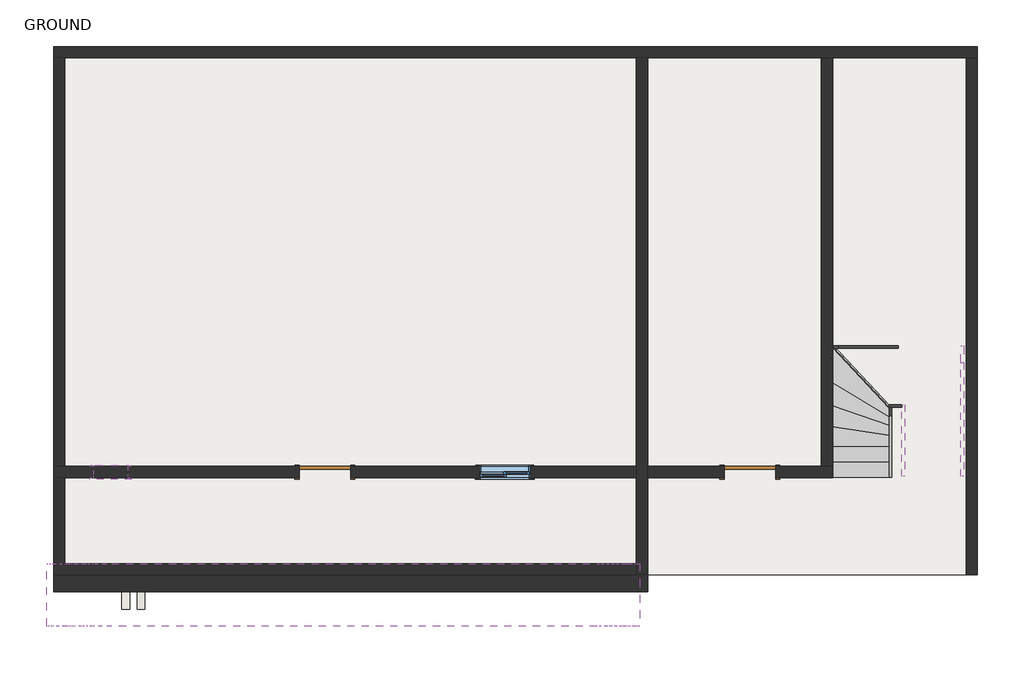
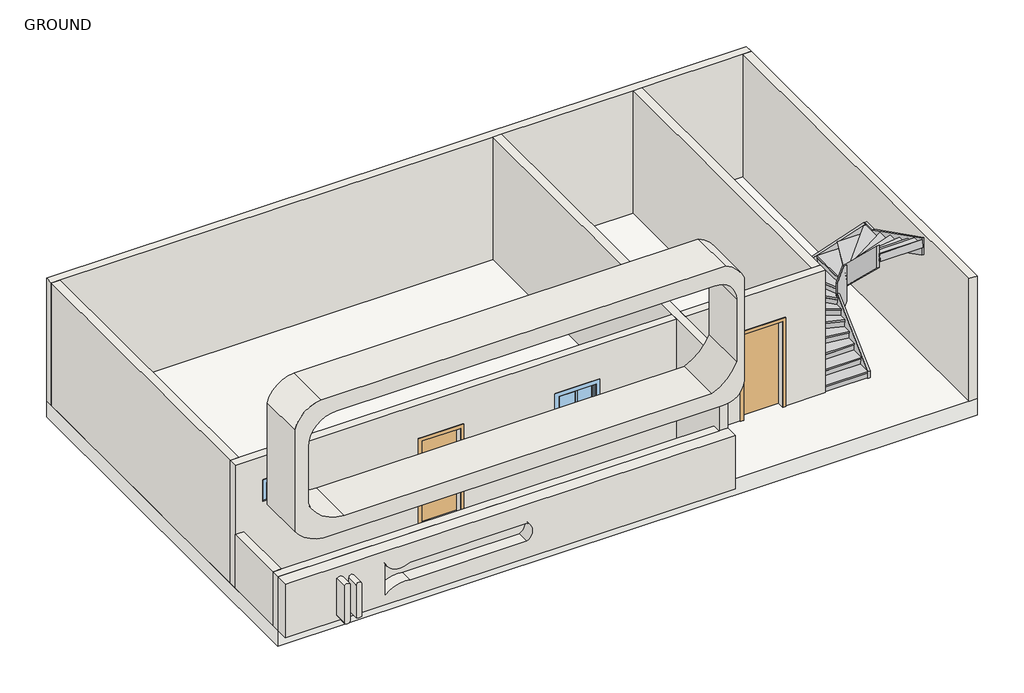
# One storey, incomplete: 12 walls, 8 members, 2 doors, 2 windows, 1 slab, 1 stair flight.
"""IFC4 building model written with IfcOpenShell, lengths in millimetres."""

from ifc_helpers import new_model, si_unit, frame, origin, origin_with_axes, place, context, project, spatial, polyline, outline, extrude, faceted_brep, transform, mapped, element, save
from components import m_single_flush_0915_x_2134mm_6a9e8738, stair_flight_50mm_tread_25mm_nosing_13mm_riser_190ae62b, walls_1_walls_1_13ff75f0, walls_4_walls_4_2d9e6e62, walls_5_walls_5_0e8582f5, window_242facca, window_372a270f

model = new_model("IFC4")

# Units and contexts
model_context = context("Model", 3, world=origin())
ifc_project = project(units=[si_unit("LENGTHUNIT", "METRE", prefix="MILLI")], contexts=[model_context])

# Site, building, storey
site = spatial("IfcSite", under=ifc_project)
building = spatial("IfcBuilding", under=site)
storey = spatial("IfcBuildingStorey", under=building, Name="GROUND", Elevation=0.0)

# Doors
placement = place(None, origin())
m_single_flush_0915_x_2134mm_shape = m_single_flush_0915_x_2134mm_6a9e8738(model_context)
element("IfcDoor", 1, ObjectType="M_Single-Flush : 0915 x 2134mm", at=placement, inside=storey, context=model_context, shape_type="MappedRepresentation", body=[
    mapped(m_single_flush_0915_x_2134mm_shape, transform((255.2261575, -1309.9510925, 0.0), x_axis=(1.0, 0.0, 0.0), y_axis=(0.0, 1.0, 0.0), z_axis=(0.0, 0.0, 1.0))),
])
element("IfcDoor", 2, ObjectType="M_Single-Flush : 0915 x 2134mm", at=placement, inside=storey, context=model_context, shape_type="MappedRepresentation", body=[
    mapped(m_single_flush_0915_x_2134mm_shape, transform((7815.0508164, -1309.9510925, 0.0), x_axis=(1.0, 0.0, 0.0), y_axis=(0.0, 1.0, 0.0), z_axis=(0.0, 0.0, 1.0))),
])

# Members
element("IfcMember", 3, ObjectType="Stringer - 50mm Width", at=placement, inside=storey, context=model_context, shape_type="SweptSolid", body=[
    extrude(outline(polyline([(-1405.5848061, 0.0), (-1405.5848061, 258.6349517), (889.7143644, 1278.8592385), (889.7143644, 841.1257613), (-1002.6491944, 0.0), (-1405.5848061, 0.0)])), frame((9239.7239729, 0.0, 0.0), z_axis=(1.0, 0.0, 0.0), x_axis=(0.0, 1.0, 0.0)), (0.0, 0.0, 1.0), 50.0),
])
element("IfcMember", 4, ObjectType="Stringer - 50mm Width", at=placement, inside=storey, context=model_context, shape_type="SweptSolid", body=[
    extrude(outline(polyline([(9239.7239729, 889.7143644), (9239.7239729, 939.7143644), (9388.2243256, 939.7143644), (9388.2243256, 889.7143644), (9239.7239729, 889.7143644)])), frame((0.0, 0.0, 841.1257613), z_axis=(0.0, 0.0, 1.0), x_axis=(1.0, 0.0, 0.0)), (0.0, 0.0, 1.0), 437.7334772),
])
element("IfcMember", 5, ObjectType="Stringer - 50mm Width", at=placement, inside=storey, context=model_context, shape_type="SweptSolid", body=[
    extrude(outline(polyline([(1278.8592385, 9388.2243256), (841.1257613, 9388.2243256), (1572.7976317, 11564.7755354), (2005.604341, 11564.7755354), (2005.604341, 11550.1195633), (1278.8592385, 9388.2243256)])), frame((0.0, 889.7143644, 0.0), z_axis=(0.0, 1.0, 0.0), x_axis=(0.0, 0.0, 1.0)), (0.0, 0.0, 1.0), 50.0),
])
element("IfcMember", 6, ObjectType="Stringer - 50mm Width", at=placement, inside=storey, context=model_context, shape_type="SweptSolid", body=[
    extrude(outline(polyline([(11564.7755354, 939.7143644), (11614.7755354, 939.7143644), (11614.7755354, 631.1318326), (11564.7755354, 631.1318326), (11564.7755354, 939.7143644)])), frame((0.0, 0.0, 1583.6082668), z_axis=(0.0, 0.0, 1.0), x_axis=(1.0, 0.0, 0.0)), (0.0, 0.0, 1.0), 421.9960743),
])
element("IfcMember", 7, ObjectType="Stringer - 50mm Width", at=placement, inside=storey, context=model_context, shape_type="SweptSolid", body=[
    extrude(outline(polyline([(631.1318326, 2005.604341), (631.1318326, 1583.6082668), (-1386.5243932, 2603.0031346), (-1386.5243932, 3024.9992088), (631.1318326, 2005.604341)])), frame((11564.7755354, 0.0, 0.0), z_axis=(1.0, 0.0, 0.0), x_axis=(0.0, 1.0, 0.0)), (0.0, 0.0, 1.0), 50.0),
])
element("IfcMember", 8, ObjectType="Stringer - 50mm Width", at=placement, inside=storey, context=model_context, shape_type="SweptSolid", body=[
    extrude(outline(polyline([(-1405.5848061, 0.0), (-1405.5848061, 167.9450175), (-160.3114169, 1349.3254446), (-160.3114169, 797.9612039), (-1001.4290028, 0.0), (-1405.5848061, 0.0)])), frame((10289.7497541, 0.0, 0.0), z_axis=(1.0, 0.0, 0.0), x_axis=(0.0, 1.0, 0.0)), (0.0, 0.0, 1.0), 50.0),
])
element("IfcMember", 9, ObjectType="Stringer - 50mm Width", at=placement, inside=storey, context=model_context, shape_type="SweptSolid", body=[
    extrude(outline(polyline([(1603.1179686, 10289.7497541), (845.3957848, 10289.7497541), (845.3957848, 10414.0648587), (1093.6297966, 10514.7497541), (1982.7346373, 10514.7497541), (1982.7346373, 10443.7240799), (1603.1179686, 10289.7497541)])), frame((0.0, -160.3114169, 0.0), z_axis=(0.0, 1.0, 0.0), x_axis=(0.0, 0.0, 1.0)), (0.0, 0.0, 1.0), 50.0),
])
element("IfcMember", 10, ObjectType="Stringer - 50mm Width", at=placement, inside=storey, context=model_context, shape_type="SweptSolid", body=[
    extrude(outline(polyline([(-110.3114169, 1982.7346373), (-110.3114169, 1429.3598105), (-1386.5243932, 2649.3941307), (-1386.5243932, 3202.7689575), (-110.3114169, 1982.7346373)])), frame((10514.7497541, 0.0, 0.0), z_axis=(1.0, 0.0, 0.0), x_axis=(0.0, 1.0, 0.0)), (0.0, 0.0, 1.0), 50.0),
])

# Slab
element("IfcSlab", 11, ObjectType="Generic Floor - 400mm", at=placement, inside=storey, context=model_context, shape_type="SweptSolid", body=[
    extrude(outline(polyline([(11861.7023789, 6257.6489075), (11861.7023789, -3138.7510925), (-4569.1738425, -3138.7510925), (-4569.1738425, 6257.6489075), (11861.7023789, 6257.6489075)])), frame((0.0, 0.0, -400.0), z_axis=(0.0, 0.0, 1.0), x_axis=(1.0, 0.0, 0.0)), (0.0, 0.0, 1.0), 400.0),
])

# Stair flight
stair_flight_50mm_tread_25mm_nosing_13mm_riser_shape = stair_flight_50mm_tread_25mm_nosing_13mm_riser_190ae62b(model_context)
element("IfcStairFlight", 12, ObjectType="50mm Tread 25mm Nosing 13mm Riser", at=placement, inside=storey, context=model_context, shape_type="MappedRepresentation", body=[
    mapped(stair_flight_50mm_tread_25mm_nosing_13mm_riser_shape, transform((0.0, 0.0, 0.0), x_axis=(1.0, 0.0, 0.0), y_axis=(0.0, 1.0, 0.0), z_axis=(0.0, 0.0, 1.0))),
])

# Walls
element("IfcWall", 13, ObjectType="Generic - 9\"", at=placement, inside=storey, context=model_context, shape_type="Brep", body=[
    faceted_brep([(-4569.1738425, 6057.6489075, 0.0), (-4369.1738425, 6057.6489075, 0.0), (5794.0261575, 6057.6489075, 0.0), (5994.0261575, 6057.6489075, 0.0), (9086.6508164, 6057.6489075, 0.0), (9286.6508164, 6057.6489075, 0.0), (11661.7023789, 6057.6489075, 0.0), (11861.7023789, 6057.6489075, 0.0), (11861.7023789, 6057.6489075, 3048.0), (11661.7023789, 6057.6489075, 3048.0), (9286.6508164, 6057.6489075, 3048.0), (9086.6508164, 6057.6489075, 3048.0), (5994.0261575, 6057.6489075, 3048.0), (5794.0261575, 6057.6489075, 3048.0), (-4369.1738425, 6057.6489075, 3048.0), (-4569.1738425, 6057.6489075, 3048.0), (-4569.1738425, 6257.6489075, 0.0), (-4569.1738425, 6257.6489075, 3048.0), (11861.7023789, 6257.6489075, 3048.0), (11861.7023789, 6257.6489075, 0.0)], [[[0, 1, 2, 3, 4, 5, 6, 7, 8, 9, 10, 11, 12, 13, 14, 15]], [[16, 17, 18, 19]], [[7, 6, 5, 4, 3, 2, 1, 0, 16, 19]], [[15, 14, 13, 12, 11, 10, 9, 8, 18, 17]], [[0, 15, 17, 16]], [[8, 7, 19, 18]]]),
])
element("IfcWall", 14, ObjectType="Generic - 9\"", at=placement, inside=storey, context=model_context, shape_type="SweptSolid", body=[
    extrude(outline(polyline([(-4569.1738425, -1209.9510925), (-4569.1738425, 6057.6489075), (-4369.1738425, 6057.6489075), (-4369.1738425, -1209.9510925), (-4569.1738425, -1209.9510925)])), origin_with_axes(), (0.0, 0.0, 1.0), 3048.0),
])
element("IfcWall", 15, ObjectType="Generic - 9\"", at=placement, inside=storey, context=model_context, shape_type="Brep", body=[
    faceted_brep([(712.7261575, -1409.9510925, 2134.0), (712.7261575, -1409.9510925, 0.0), (5794.0261575, -1409.9510925, 0.0), (5794.0261575, -1409.9510925, 3048.0), (-4569.1738425, -1409.9510925, 3048.0), (-4569.1738425, -1409.9510925, 1329.6628337), (-4569.1738425, -1409.9510925, 0.0), (-4369.1738425, -1409.9510925, 0.0), (-202.2738425, -1409.9510925, 0.0), (-202.2738425, -1409.9510925, 2134.0), (2998.4261575, -1409.9510925, 2133.6), (3912.8261575, -1409.9510925, 2133.6), (3912.8261575, -1409.9510925, 914.4), (2998.4261575, -1409.9510925, 914.4), (-3859.5738425, -1409.9510925, 2399.5080367), (-3249.9738425, -1409.9510925, 2399.5080367), (-3249.9738425, -1409.9510925, 1942.3080367), (-3859.5738425, -1409.9510925, 1942.3080367), (5794.0261575, -1209.9510925, 0.0), (712.7261575, -1209.9510925, 0.0), (712.7261575, -1209.9510925, 2134.0), (-202.2738425, -1209.9510925, 2134.0), (-202.2738425, -1209.9510925, 0.0), (-4369.1738425, -1209.9510925, 0.0), (-4569.1738425, -1209.9510925, 0.0), (-4569.1738425, -1209.9510925, 3048.0), (-4369.1738425, -1209.9510925, 3048.0), (5794.0261575, -1209.9510925, 3048.0), (2998.4261575, -1209.9510925, 2133.6), (2998.4261575, -1209.9510925, 914.4), (3912.8261575, -1209.9510925, 914.4), (3912.8261575, -1209.9510925, 2133.6), (-3859.5738425, -1209.9510925, 2399.5080367), (-3859.5738425, -1209.9510925, 1942.3080367), (-3249.9738425, -1209.9510925, 1942.3080367), (-3249.9738425, -1209.9510925, 2399.5080367)], [[[0, 1, 2, 3, 4, 5, 6, 7, 8, 9], [10, 11, 12, 13], [14, 15, 16, 17]], [[18, 19, 20, 21, 22, 23, 24, 25, 26, 27], [28, 29, 30, 31], [32, 33, 34, 35]], [[2, 1, 19, 18]], [[8, 7, 6, 24, 23, 22]], [[4, 3, 27, 26, 25]], [[3, 2, 18, 27]], [[20, 19, 1, 0]], [[21, 20, 0, 9]], [[22, 21, 9, 8]], [[29, 28, 10, 13]], [[30, 29, 13, 12]], [[31, 30, 12, 11]], [[28, 31, 11, 10]], [[4, 25, 24, 6, 5]], [[33, 32, 14, 17]], [[34, 33, 17, 16]], [[35, 34, 16, 15]], [[32, 35, 15, 14]]]),
])
element("IfcWall", 16, ObjectType="Generic - 9\"", at=placement, inside=storey, context=model_context, shape_type="SweptSolid", body=[
    extrude(outline(polyline([(11861.7023789, 6057.6489075), (11861.7023789, -3138.7510925), (11661.7023789, -3138.7510925), (11661.7023789, 6057.6489075), (11861.7023789, 6057.6489075)])), origin_with_axes(), (0.0, 0.0, 1.0), 3048.0),
])
element("IfcWall", 17, ObjectType="Generic - 9\"", at=placement, inside=storey, context=model_context, shape_type="Brep", body=[
    faceted_brep([(5794.0261575, 6057.6489075, 0.0), (5794.0261575, -1209.9510925, 0.0), (5794.0261575, -1409.9510925, 0.0), (5794.0261575, -2938.7510925, 0.0), (5794.0261575, -3138.7510925, 0.0), (5794.0261575, -3138.7510925, 1323.5671837), (5794.0261575, -3138.7510925, 3048.0), (5794.0261575, -1409.9510925, 3048.0), (5794.0261575, -1209.9510925, 3048.0), (5794.0261575, 6057.6489075, 3048.0), (5994.0261575, 6057.6489075, 0.0), (5994.0261575, 6057.6489075, 3048.0), (5994.0261575, -1209.9510925, 3048.0), (5994.0261575, -1409.9510925, 3048.0), (5994.0261575, -3138.7510925, 3048.0), (5994.0261575, -3138.7510925, 0.0), (5994.0261575, -1409.9510925, 0.0), (5994.0261575, -1209.9510925, 0.0)], [[[0, 1, 2, 3, 4, 5, 6, 7, 8, 9]], [[10, 11, 12, 13, 14, 15, 16, 17]], [[4, 3, 2, 1, 0, 10, 17, 16, 15]], [[9, 8, 7, 6, 14, 13, 12, 11]], [[0, 9, 11, 10]], [[6, 5, 4, 15, 14]]]),
])
element("IfcWall", 18, ObjectType="Generic - 9\"", at=placement, inside=storey, context=model_context, shape_type="Brep", body=[
    faceted_brep([(9286.6508164, -1209.9510925, 0.0), (9086.6508164, -1209.9510925, 0.0), (8272.5508164, -1209.9510925, 0.0), (8272.5508164, -1209.9510925, 2134.0), (7357.5508164, -1209.9510925, 2134.0), (7357.5508164, -1209.9510925, 0.0), (5994.0261575, -1209.9510925, 0.0), (5994.0261575, -1209.9510925, 3048.0), (9086.6508164, -1209.9510925, 3048.0), (9286.6508164, -1209.9510925, 3048.0), (8272.5508164, -1409.9510925, 2134.0), (8272.5508164, -1409.9510925, 0.0), (9286.6508164, -1409.9510925, 0.0), (9286.6508164, -1409.9510925, 3048.0), (5994.0261575, -1409.9510925, 3048.0), (5994.0261575, -1409.9510925, 0.0), (7357.5508164, -1409.9510925, 0.0), (7357.5508164, -1409.9510925, 2134.0)], [[[0, 1, 2, 3, 4, 5, 6, 7, 8, 9]], [[10, 11, 12, 13, 14, 15, 16, 17]], [[16, 15, 6, 5]], [[12, 11, 2, 1, 0]], [[9, 8, 7, 14, 13]], [[0, 9, 13, 12]], [[7, 6, 15, 14]], [[3, 2, 11, 10]], [[4, 3, 10, 17]], [[5, 4, 17, 16]]]),
])
element("IfcWall", 19, ObjectType="Generic - 9\"", at=placement, inside=storey, context=model_context, shape_type="SweptSolid", body=[
    extrude(outline(polyline([(9086.6508164, -1209.9510925), (9086.6508164, 6057.6489075), (9286.6508164, 6057.6489075), (9286.6508164, -1209.9510925), (9086.6508164, -1209.9510925)])), origin_with_axes(), (0.0, 0.0, 1.0), 3048.0),
])
element("IfcWall", 20, ObjectType="Generic - 9\"", at=placement, inside=storey, context=model_context, shape_type="Brep", body=[
    faceted_brep([(5794.0261575, -2938.7510925, 0.0), (-4369.1738425, -2938.7510925, 0.0), (-4569.1738425, -2938.7510925, 0.0), (-4569.1738425, -2938.7510925, 1323.5671837), (5794.0261575, -2938.7510925, 1323.5671837), (5794.0261575, -3138.7510925, 0.0), (5794.0261575, -3138.7510925, 1323.5671837), (-4569.1738425, -3138.7510925, 1323.5671837), (-4569.1738425, -3138.7510925, 0.0)], [[[0, 1, 2, 3, 4]], [[5, 6, 7, 8]], [[2, 1, 0, 5, 8]], [[4, 3, 7, 6]], [[0, 4, 6, 5]], [[3, 2, 8, 7]]]),
])
element("IfcWall", 21, ObjectType="Generic - 9\"", at=placement, inside=storey, context=model_context, shape_type="Brep", body=[
    faceted_brep([(-4569.1738425, -1409.9510925, 0.0), (-4569.1738425, -2938.7510925, 0.0), (-4569.1738425, -2938.7510925, 1323.5671837), (-4569.1738425, -2938.7510925, 1329.6628337), (-4569.1738425, -1409.9510925, 1329.6628337), (-4369.1738425, -1409.9510925, 0.0), (-4369.1738425, -1409.9510925, 1329.6628337), (-4369.1738425, -2938.7510925, 1329.6628337), (-4369.1738425, -2938.7510925, 0.0)], [[[0, 1, 2, 3, 4]], [[5, 6, 7, 8]], [[1, 0, 5, 8]], [[4, 3, 7, 6]], [[0, 4, 6, 5]], [[3, 2, 1, 8, 7]]]),
])
walls_1_walls_1_shape = walls_1_walls_1_13ff75f0(model_context)
element("IfcWall", 22, ObjectType="Walls 1 : Walls 1", at=placement, inside=storey, context=model_context, shape_type="MappedRepresentation", body=[
    mapped(walls_1_walls_1_shape, transform((0.0, 0.0, 0.0), x_axis=(1.0, 0.0, 0.0), y_axis=(0.0, 1.0, 0.0), z_axis=(0.0, 0.0, 1.0))),
])
walls_4_walls_4_shape = walls_4_walls_4_2d9e6e62(model_context)
element("IfcWall", 23, ObjectType="Walls 4 : Walls 4", at=placement, inside=storey, context=model_context, shape_type="MappedRepresentation", body=[
    mapped(walls_4_walls_4_shape, transform((0.0, 0.0, 0.0), x_axis=(1.0, 0.0, 0.0), y_axis=(0.0, 1.0, 0.0), z_axis=(0.0, 0.0, 1.0))),
])
walls_5_walls_5_shape = walls_5_walls_5_0e8582f5(model_context)
element("IfcWall", 24, ObjectType="Walls 5 : Walls 5", at=placement, inside=storey, context=model_context, shape_type="MappedRepresentation", body=[
    mapped(walls_5_walls_5_shape, transform((0.0, 0.0, 0.0), x_axis=(1.0, 0.0, 0.0), y_axis=(0.0, 1.0, 0.0), z_axis=(0.0, 0.0, 1.0))),
])

# Windows
window_shape = window_242facca(model_context)
element("IfcWindow", 25, ObjectType="Slider with Trim : 36\" x 48\"", at=placement, inside=storey, context=model_context, shape_type="MappedRepresentation", body=[
    mapped(window_shape, transform((3455.6261575, -1309.9510925, 0.0), x_axis=(-1.0, 0.0, 0.0), y_axis=(0.0, -1.0, 0.0), z_axis=(0.0, 0.0, 1.0))),
])
window_2_shape = window_372a270f(model_context)
element("IfcWindow", 26, ObjectType="Transom with Trim : 24\" x 18\"", at=placement, inside=storey, context=model_context, shape_type="MappedRepresentation", body=[
    mapped(window_2_shape, transform((-3592.8738425, -1309.9510925, -216.6919633), x_axis=(-1.0, 0.0, 0.0), y_axis=(0.0, -1.0, 0.0), z_axis=(0.0, 0.0, 1.0))),
])

save(model, "model.ifc")

# Revit data of these elements
# Type "M_Single-Flush : 0915 x 2134mm"
#   Type Mark = "15"
#   Thickness = 0' - 2.00787"
#   Height = 7' - 0.01575"
#   Trim Projection Ext = 0' - 0.98425"
#   Trim Projection Int = 0' - 0.98425"
#   Trim Width = 0' - 2.99213"
#   Width = 3' - 0.02362"
#   Door Material = Door - Panel
#   Frame Material = Door - Frame
#   Function = (empty or 0)
#   Wall Closure = (empty or 0)
# Type "Generic Floor - 400mm"
#   Function = 0
#   Layers, outside or top first: 1' - 3.74803" no material (function 1)
# Type "Generic - 9\""
#   Layers, outside or top first: 0' - 7.87402" no material (function 1)
# Type "Slider with Trim : 36\" x 48\""
#   Type Mark = "19"
#   Construction Type Id = "GSP4R"
#   Assembly Code = "B2020100"
#   Analytic Construction = "1/8 in Pilkington single glazing"
#   Visual Light Transmittance = 0.9
#   Solar Heat Gain Coefficient = 0.78
#   Heat Transfer Coefficient (U) = 3.6886 W/(m²·K)
#   Height = 4' - 0"
#   Default Sill Height = 3' - 0"
#   Trim Projection - Ext. = 0' - 0 3/4"
#   Trim Projection - Int. = 0' - 0 3/4"
#   Trim Width - Exterior = 0' - 3 1/2"
#   Trim Width - Interior = 0' - 3 1/2"
#   Width = 3' - 0"
#   Window Inset = 0' - 0 3/4"
#   Define Thermal Properties by = 1
#   Glass Pane Material = Glass
#   Sash Material = Sash
#   Trim Exterior Material = Trim
#   Trim Interior Material = Trim
#   Wall Closure = (empty or 0)
# Type "Transom with Trim : 24\" x 18\""
#   Type Mark = "30"
#   Construction Type Id = "GSP4R"
#   Assembly Code = "B2020100"
#   Analytic Construction = "1/8 in Pilkington single glazing"
#   Visual Light Transmittance = 0.9
#   Solar Heat Gain Coefficient = 0.78
#   Heat Transfer Coefficient (U) = 3.6886 W/(m²·K)
#   Height = 1' - 6"
#   Default Sill Height = 7' - 1"
#   Trim Projection - Ext. = 0' - 0 1/2"
#   Trim Projection - Int. = 0' - 0 3/4"
#   Trim Width - Exterior = 0' - 3 1/2"
#   Trim Width - Interior = 0' - 3 1/2"
#   Width = 2' - 0"
#   Window Inset = 0' - 0 3/4"
#   Define Thermal Properties by = 1
#   Glass Pane Material = Glass
#   Sash Material = Sash
#   Trim Exterior Material = Trim
#   Trim Interior Material = Trim
#   Wall Closure = (empty or 0)
# Elements 1, 2 (IfcDoor, "M_Single-Flush : 0915 x 2134mm")
#   Phase Created = New Construction
#   Materials on its faces: "Door - Frame", "Door - Panel"
# Elements 3, 4, 5, 6, 7, 8, 9, 10 (IfcMember, "Stringer - 50mm Width")
#   Phase Created = New Construction
# Element 11 (IfcSlab, "Generic Floor - 400mm")
#   Height Offset From Level = 0' - 0"
#   Phase Created = New Construction
#   Materials on its faces: "Default Roof"
# Element 12 (IfcStairFlight, "50mm Tread 25mm Nosing 13mm Riser")
#   Phase Created = New Construction
# Elements 13, 14, 15, 16, 17, 18, 19 (IfcWall, "Generic - 9\"")
#   Top Offset = 0' - 0"
#   Base Offset = 0' - 0"
#   Unconnected Height = 10' - 0"
#   wall height = 10' - 0"
#   Phase Created = New Construction
#   Base Constraint = GROUND
#   Materials on its faces: "Default Wall"
# Element 20 (IfcWall, "Generic - 9\"")
#   Top Offset = 0' - 0"
#   Base Offset = 0' - 0"
#   Unconnected Height = 4' - 4.10894"
#   wall height = 4' - 4.10894"
#   Phase Created = New Construction
#   Base Constraint = GROUND
#   Materials on its faces: "Default Wall"
# Element 21 (IfcWall, "Generic - 9\"")
#   Top Offset = 0' - 0"
#   Base Offset = 0' - 0"
#   Unconnected Height = 4' - 4.34893"
#   wall height = 4' - 4.34893"
#   Phase Created = New Construction
#   Base Constraint = GROUND
#   Materials on its faces: "Default Wall"
# Element 22 (IfcWall, "Walls 1 : Walls 1")
#   Phase Created = New Construction
#   Materials on its faces: "Default Wall"
# Element 23 (IfcWall, "Walls 4 : Walls 4")
#   Phase Created = New Construction
#   Materials on its faces: "Default Wall"
# Element 24 (IfcWall, "Walls 5 : Walls 5")
#   Phase Created = New Construction
#   Materials on its faces: "Default Wall"
# Element 25 (IfcWindow, "Slider with Trim : 36\" x 48\"")
#   Mark = "6"
#   Phase Created = New Construction
#   Materials on its faces: "Sash", "Trim", "Glass"
# Element 26 (IfcWindow, "Transom with Trim : 24\" x 18\"")
#   Mark = "12"
#   Phase Created = New Construction
#   Materials on its faces: "Sash", "Trim", "Glass"
# Materials
#   "Door - Panel": class "Wood", colour RGB 114 82 51, transparency 0
#   "Door - Frame": colour RGB 153 76 43, transparency 0
#   "Glass": class "Glass", colour RGB 218 227 224, transparency 0.85, Description = "Soda Lime Glass", Cost = 0
#   "Sash": class "Wood", colour RGB 136 99 55, transparency 0
#   "Trim": class "Wood", colour RGB 224 178 126, transparency 0
#   "Default Roof": colour RGB 80 80 80, transparency 0
#   "Default Wall": colour RGB 80 80 80, transparency 0
